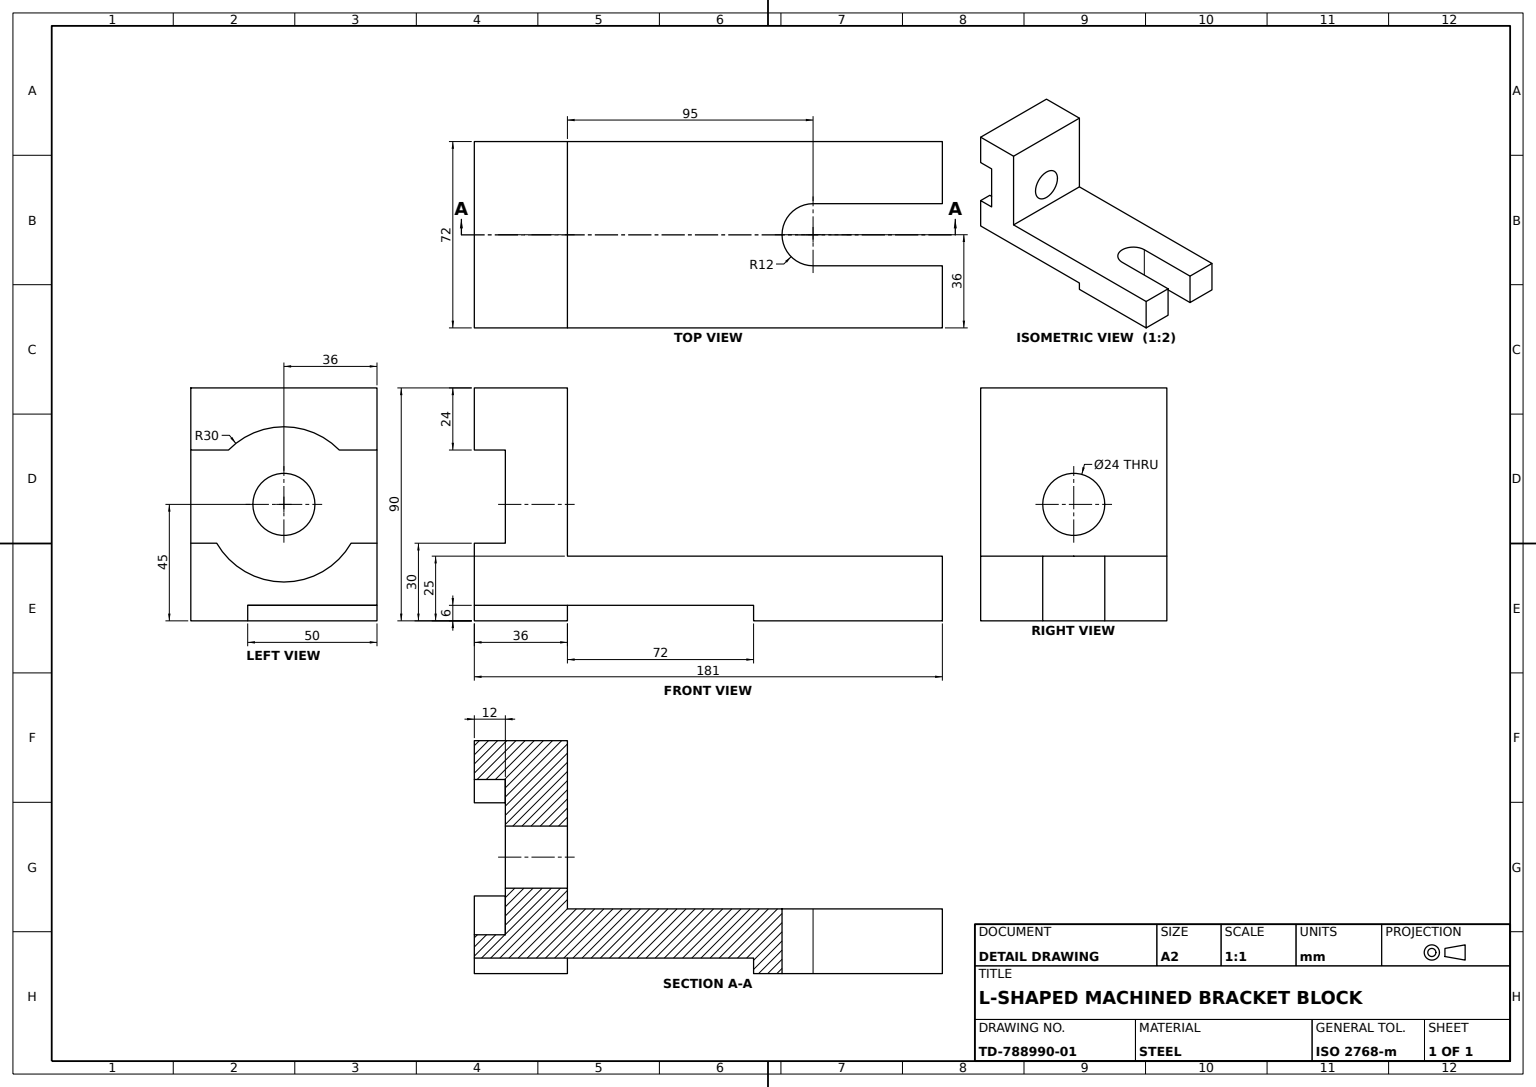
from build123d import *

# Parameters (mm, degrees)
BASE_BLOCK_SKETCH_W       = 72
BASE_BLOCK_SKETCH_H       = 90
BASE_BLOCK_90X72X36_DEPTH = 18
ARC_RECESS_SKETCH_R       = 30
ARC_RECESS_60_DEPTH       = 12
BORE_24_DEPTH             = 117.653332571
RECESS_RELIEF_SKETCH_R    = 12
RECESS_RELIEF_CUT_DEPTH   = 118.728501222
BOTTOM_GROOVE_SKETCH_W    = 50
BOTTOM_GROOVE_SKETCH_H    = 6
BOTTOM_GROOVE_6X50_DEPTH  = 121.747670785
FORK_ARM_DEPTH            = 72
FORK_SLOT_24_DEPTH        = 190.67867566


with BuildPart() as part:
    # Base Block Sketch → Base Block 90x72x36 (new, symmetric)
    with BuildSketch(Plane.XY):
        with Locations((36, 45)):
            Rectangle(BASE_BLOCK_SKETCH_W, BASE_BLOCK_SKETCH_H)
    extrude(amount=BASE_BLOCK_90X72X36_DEPTH, both=True)

    # Arc Recess Sketch → Arc Recess Ø60 (cut)
    with BuildSketch(Plane.XY.offset(18)):
        with Locations((36, 45)):
            Circle(ARC_RECESS_SKETCH_R)
    extrude(amount=-ARC_RECESS_60_DEPTH, mode=Mode.SUBTRACT)

    # Bore Sketch → Bore Ø24 (cut, through all)
    with BuildSketch(Plane(origin=(72, 0, 0), x_dir=(0, 0, -1), z_dir=(1, 0, 0))):
        Polygon((-18, 66), (-6, 66), (-6, 45), (-6, 30), (-18, 30), align=None)
    extrude(amount=-BORE_24_DEPTH, mode=Mode.SUBTRACT)

    # Recess Relief Sketch → Recess Relief Cut (cut, through all)
    with BuildSketch(Plane.XY.offset(6)):
        with Locations((36, 45)):
            Circle(RECESS_RELIEF_SKETCH_R)
    extrude(amount=-RECESS_RELIEF_CUT_DEPTH, mode=Mode.SUBTRACT)

    # Bottom Groove Sketch → Bottom Groove 6x50 (cut, through all)
    with BuildSketch(Plane.XY.offset(18)):
        with Locations((47, 3)):
            Rectangle(BOTTOM_GROOVE_SKETCH_W, BOTTOM_GROOVE_SKETCH_H)
    extrude(amount=-BOTTOM_GROOVE_6X50_DEPTH, mode=Mode.SUBTRACT)

    # Fork Arm Sketch → Fork Arm (add)
    with BuildSketch(Plane(origin=(72, 0, 0), x_dir=(0, 0, -1), z_dir=(1, 0, 0))):
        Polygon((18, 6), (90, 6), (90, 0), (163, 0), (163, 25), (18, 25), align=None)
    extrude(amount=-FORK_ARM_DEPTH)

    # Fork Slot Sketch → Fork Slot 24 (cut, through all)
    with BuildSketch(Plane(origin=(0, 25, 0), x_dir=(1, 0, 0), z_dir=(0, 1, 0))):
        with BuildLine():
            Line((48, 163), (48, 113))
            ThreePointArc((48, 113), (36, 101), (24, 113))
            Line((24, 113), (24, 163))
            Line((24, 163), (48, 163))
        make_face()
    extrude(amount=-FORK_SLOT_24_DEPTH, mode=Mode.SUBTRACT)


solid = part.part
